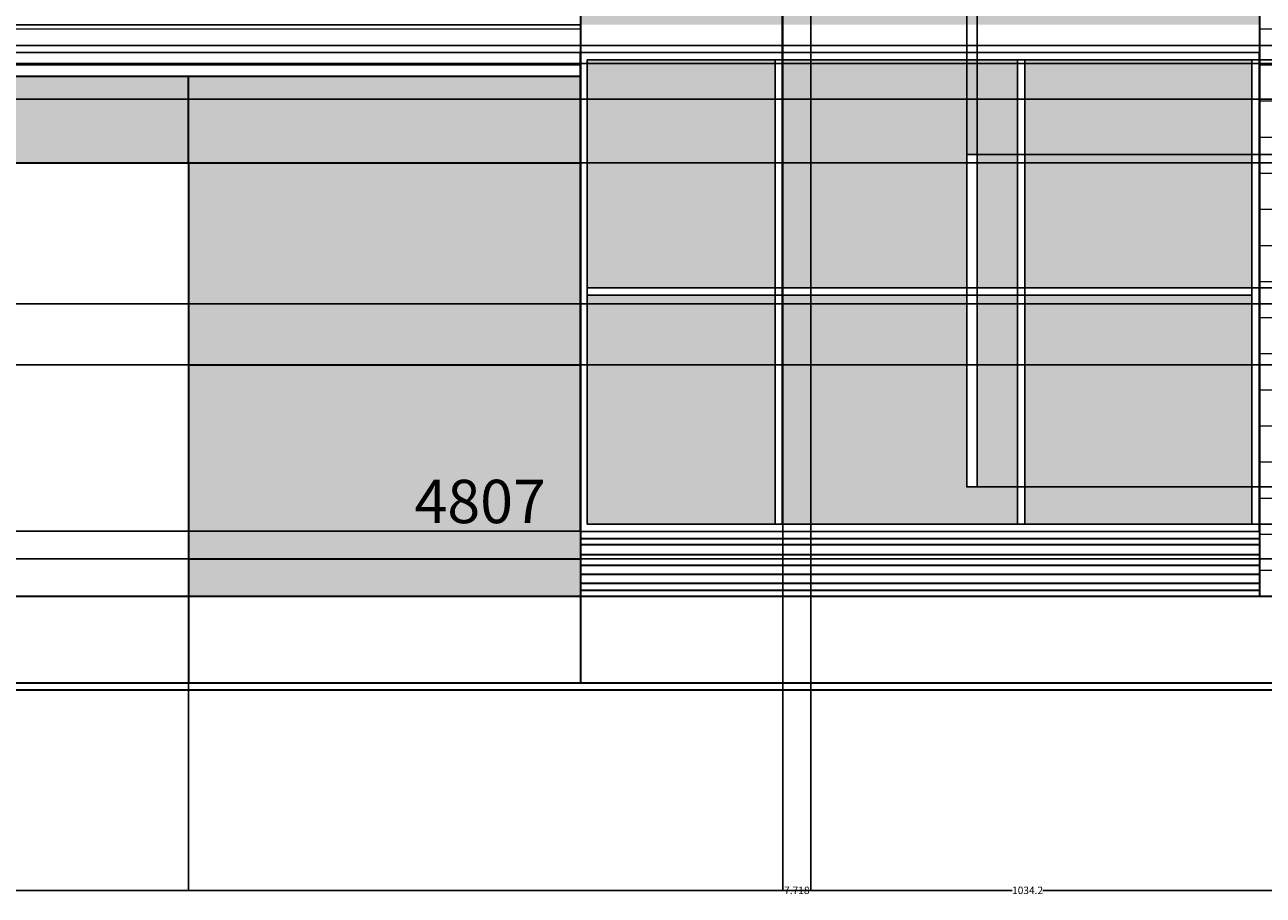
# Model space of a CAD drawing. Units: inches. Extents: x -30 to 1188, y 40 to 520.
# Tile 3 of 7: x 313 to 656, y 40 to 281. Entities that reach past the tile are written whole.
import ezdxf

# ---------------------------------------------------------------- set-up
doc = ezdxf.new("R2010")
doc.units = ezdxf.units.IN
doc.header["$MEASUREMENT"] = 0
for name, color, linetype, lineweight in [('A-ANNO-DIMS', 2, 'Continuous', 18), ('A-ANNO-TEXT', 7, 'Continuous', 25), ('A-DOOR', 3, 'Continuous', 25), ('A-ELEV', 7, 'Continuous', 35), ('A-ELEV-PATT', 8, 'Continuous', 13)]:
    doc.layers.add(name, color=color, linetype=linetype, lineweight=lineweight)
doc.styles.get("Standard").update_dxf_attribs({"font": 'arial.ttf'})
doc.dimstyles.get("Standard").update_dxf_attribs({"dimtxt": 2.0625, "dimasz": 0.18, "dimexe": 0.18, "dimexo": 0.0625, "dimgap": 0.09, "dimtad": 0, "dimtih": 1, "dimtoh": 1, "dimdec": 4, "dimzin": 0, "dimdsep": 46, "dimlunit": 4, "dimtxsty": 'Standard', "dimcen": 0.09, "dimadec": 0, "dimazin": 0, "dimtfac": 1, "dimtdec": 4, "dimtofl": 0, "dimtmove": 0, "dimatfit": 3, "dimfxl": 1, "dimtolj": 1, "dimtzin": 0, "dimarcsym": 0})

# ---------------------------------------------------------------- blocks, each defined once
blk = doc.blocks.new('*D4')
at = {"layer": 'A-ANNO-DIMS', "color": 0, "lineweight": -2, "transparency": 16777216}
for p, q in [((73.66, 122.81), (73.66, 41.19)), ((1107.88, 118.31), (1107.88, 41.19)), ((73.84, 41.37), (586.5, 41.37)), ((1107.7, 41.37), (595.03, 41.37))]:
    blk.add_line(p, q, dxfattribs=at)
at = {"layer": 'A-ANNO-DIMS', "color": 0, "transparency": 16777216}
for points in [[(73.84, 41.4), (73.84, 41.34), (73.66, 41.37)], [(1107.7, 41.4), (1107.7, 41.34), (1107.88, 41.37)]]:
    blk.add_solid(points, dxfattribs=at)
at = {"layer": 'Defpoints', "color": 0, "transparency": 16777216}
for p in [(73.66, 122.87), (1107.88, 118.38), (1107.88, 41.37)]:
    blk.add_point(p, dxfattribs=at)
at = {"layer": 'A-ANNO-DIMS', "color": 0, "transparency": 16777216, "insert": (590.77, 41.37), "char_height": 2.062, "attachment_point": 5}
blk.add_mtext('\\A1;1034.2', dxfattribs=at)
blk = doc.blocks.new('*D9')
at = {"layer": 'A-ANNO-DIMS', "color": 0, "lineweight": -2, "transparency": 16777216}
for p, q in [((99.43, 98.81), (99.43, 41.19)), ((358.42, 98.81), (358.42, 41.19)), ((99.61, 41.37), (226.54, 41.37)), ((358.24, 41.37), (231.32, 41.37))]:
    blk.add_line(p, q, dxfattribs=at)
at = {"layer": 'A-ANNO-DIMS', "color": 0, "transparency": 16777216}
for points in [[(99.61, 41.4), (99.61, 41.34), (99.43, 41.37)], [(358.24, 41.4), (358.24, 41.34), (358.42, 41.37)]]:
    blk.add_solid(points, dxfattribs=at)
at = {"layer": 'Defpoints', "color": 0, "transparency": 16777216}
for p in [(99.43, 98.87), (358.42, 98.87), (358.42, 41.37)]:
    blk.add_point(p, dxfattribs=at)
at = {"layer": 'A-ANNO-DIMS', "color": 0, "transparency": 16777216, "insert": (228.93, 41.37), "char_height": 2.062, "attachment_point": 5}
blk.add_mtext('\\A1;259', dxfattribs=at)
blk = doc.blocks.new('*D20')
at = {"layer": 'A-ANNO-DIMS', "color": 0, "lineweight": -2, "transparency": 16777216}
for p, q in [((358.36, 242.87), (-25.83, 242.87)), ((-25.65, 242.69), (-25.65, 172)), ((-25.65, 99.05), (-25.65, 169.75)), ((358.36, 98.87), (-25.83, 98.87))]:
    blk.add_line(p, q, dxfattribs=at)
at = {"layer": 'A-ANNO-DIMS', "color": 0, "transparency": 16777216}
for points in [[(-25.68, 242.69), (-25.62, 242.69), (-25.65, 242.87)], [(-25.68, 99.05), (-25.62, 99.05), (-25.65, 98.87)]]:
    blk.add_solid(points, dxfattribs=at)
at = {"layer": 'Defpoints', "color": 0, "transparency": 16777216}
for p in [(-25.65, 242.87), (358.42, 242.87), (358.42, 98.87)]:
    blk.add_point(p, dxfattribs=at)
at = {"layer": 'A-ANNO-DIMS', "color": 0, "transparency": 16777216, "insert": (-25.65, 170.87), "char_height": 2.062, "attachment_point": 5}
blk.add_mtext('\\A1;144', dxfattribs=at)
blk = doc.blocks.new('*D29')
at = {"layer": 'A-ANNO-DIMS', "color": 0, "lineweight": -2, "transparency": 16777216}
for p, q in [((792.57, 270.37), (-25.83, 270.37)), ((-25.65, 270.19), (-25.65, 238.25)), ((-25.65, 204.02), (-25.65, 235.96)), ((792.57, 203.84), (-25.83, 203.84))]:
    blk.add_line(p, q, dxfattribs=at)
at = {"layer": 'A-ANNO-DIMS', "color": 0, "transparency": 16777216}
for points in [[(-25.68, 270.19), (-25.62, 270.19), (-25.65, 270.37)], [(-25.68, 204.02), (-25.62, 204.02), (-25.65, 203.84)]]:
    blk.add_solid(points, dxfattribs=at)
at = {"layer": 'Defpoints', "color": 0, "transparency": 16777216}
for p in [(-25.65, 270.37), (792.63, 270.37), (792.63, 203.84)]:
    blk.add_point(p, dxfattribs=at)
at = {"layer": 'A-ANNO-DIMS', "color": 0, "transparency": 16777216, "insert": (-25.65, 237.11), "char_height": 2.062, "attachment_point": 5}
blk.add_mtext('\\A1;66.53', dxfattribs=at)
blk = doc.blocks.new('*D31')
at = {"layer": 'A-ANNO-DIMS', "color": 0, "lineweight": -2, "transparency": 16777216}
for p, q in [((792.57, 203.84), (-25.83, 203.84)), ((-25.65, 203.66), (-25.65, 164.5)), ((-25.65, 123.05), (-25.65, 162.21)), ((935.84, 122.87), (-25.83, 122.87))]:
    blk.add_line(p, q, dxfattribs=at)
at = {"layer": 'A-ANNO-DIMS', "color": 0, "transparency": 16777216}
for points in [[(-25.68, 203.66), (-25.62, 203.66), (-25.65, 203.84)], [(-25.68, 123.05), (-25.62, 123.05), (-25.65, 122.87)]]:
    blk.add_solid(points, dxfattribs=at)
at = {"layer": 'Defpoints', "color": 0, "transparency": 16777216}
for p in [(792.63, 203.84), (-25.65, 122.87), (935.9, 122.87)]:
    blk.add_point(p, dxfattribs=at)
at = {"layer": 'A-ANNO-DIMS', "color": 0, "transparency": 16777216, "insert": (-25.65, 163.36), "char_height": 2.062, "attachment_point": 5}
blk.add_mtext('\\A1;80.97', dxfattribs=at)
blk = doc.blocks.new('*D35')
at = {"layer": 'A-ANNO-DIMS', "color": 0, "lineweight": -2, "transparency": 16777216}
for p, q in [((99.49, 122.87), (1183.93, 122.87)), ((1183.75, 122.69), (1183.75, 112)), ((1183.75, 99.05), (1183.75, 109.75)), ((99.49, 98.87), (1183.93, 98.87))]:
    blk.add_line(p, q, dxfattribs=at)
at = {"layer": 'A-ANNO-DIMS', "color": 0, "transparency": 16777216}
for points in [[(1183.72, 122.69), (1183.78, 122.69), (1183.75, 122.87)], [(1183.72, 99.05), (1183.78, 99.05), (1183.75, 98.87)]]:
    blk.add_solid(points, dxfattribs=at)
at = {"layer": 'Defpoints', "color": 0, "transparency": 16777216}
for p in [(99.43, 122.87), (1183.75, 122.87), (99.43, 98.87)]:
    blk.add_point(p, dxfattribs=at)
at = {"layer": 'A-ANNO-DIMS', "color": 0, "transparency": 16777216, "insert": (1183.75, 110.87), "char_height": 2.062, "attachment_point": 5}
blk.add_mtext('\\A1;24', dxfattribs=at)
blk = doc.blocks.new('*D36')
at = {"layer": 'A-ANNO-DIMS', "color": 0, "lineweight": -2, "transparency": 16777216}
for p, q in [((99.49, 133.14), (1183.93, 133.14)), ((1183.75, 132.96), (1183.75, 129.15)), ((1183.75, 123.05), (1183.75, 126.86)), ((99.49, 122.87), (1183.93, 122.87))]:
    blk.add_line(p, q, dxfattribs=at)
at = {"layer": 'A-ANNO-DIMS', "color": 0, "transparency": 16777216}
for points in [[(1183.72, 132.96), (1183.78, 132.96), (1183.75, 133.14)], [(1183.72, 123.05), (1183.78, 123.05), (1183.75, 122.87)]]:
    blk.add_solid(points, dxfattribs=at)
at = {"layer": 'Defpoints', "color": 0, "transparency": 16777216}
for p in [(99.43, 133.14), (1183.75, 133.14), (99.43, 122.87)]:
    blk.add_point(p, dxfattribs=at)
at = {"layer": 'A-ANNO-DIMS', "color": 0, "transparency": 16777216, "insert": (1183.75, 128.01), "char_height": 2.062, "attachment_point": 5}
blk.add_mtext('\\A1;10.268', dxfattribs=at)
blk = doc.blocks.new('*D37')
at = {"layer": 'A-ANNO-DIMS', "color": 0, "lineweight": -2, "transparency": 16777216}
for p, q in [((99.49, 186.93), (1183.93, 186.93)), ((1183.75, 186.75), (1183.75, 161.18)), ((1183.75, 133.32), (1183.75, 158.89)), ((99.49, 133.14), (1183.93, 133.14))]:
    blk.add_line(p, q, dxfattribs=at)
at = {"layer": 'A-ANNO-DIMS', "color": 0, "transparency": 16777216}
for points in [[(1183.72, 186.75), (1183.78, 186.75), (1183.75, 186.93)], [(1183.72, 133.32), (1183.78, 133.32), (1183.75, 133.14)]]:
    blk.add_solid(points, dxfattribs=at)
at = {"layer": 'Defpoints', "color": 0, "transparency": 16777216}
for p in [(99.43, 186.93), (1183.75, 186.93), (99.43, 133.14)]:
    blk.add_point(p, dxfattribs=at)
at = {"layer": 'A-ANNO-DIMS', "color": 0, "transparency": 16777216, "insert": (1183.75, 160.03), "char_height": 2.062, "attachment_point": 5}
blk.add_mtext('\\A1;53.79', dxfattribs=at)
blk = doc.blocks.new('*D38')
at = {"layer": 'A-ANNO-DIMS', "color": 0, "lineweight": -2, "transparency": 16777216}
for p, q in [((99.49, 242.87), (1183.93, 242.87)), ((1183.75, 242.69), (1183.75, 216.04)), ((1183.75, 187.11), (1183.75, 213.76)), ((99.49, 186.93), (1183.93, 186.93))]:
    blk.add_line(p, q, dxfattribs=at)
at = {"layer": 'A-ANNO-DIMS', "color": 0, "transparency": 16777216}
for points in [[(1183.72, 242.69), (1183.78, 242.69), (1183.75, 242.87)], [(1183.72, 187.11), (1183.78, 187.11), (1183.75, 186.93)]]:
    blk.add_solid(points, dxfattribs=at)
at = {"layer": 'Defpoints', "color": 0, "transparency": 16777216}
for p in [(99.43, 242.87), (1183.75, 242.87), (99.43, 186.93)]:
    blk.add_point(p, dxfattribs=at)
at = {"layer": 'A-ANNO-DIMS', "color": 0, "transparency": 16777216, "insert": (1183.75, 214.9), "char_height": 2.062, "attachment_point": 5}
blk.add_mtext('\\A1;55.94', dxfattribs=at)
blk = doc.blocks.new('*D39')
at = {"layer": 'A-ANNO-DIMS', "color": 0, "lineweight": -2, "transparency": 16777216}
for p, q in [((358.49, 186.93), (1183.93, 186.93)), ((1183.75, 186.75), (1183.75, 161.18)), ((1183.75, 133.32), (1183.75, 158.89)), ((358.49, 133.14), (1183.93, 133.14))]:
    blk.add_line(p, q, dxfattribs=at)
at = {"layer": 'A-ANNO-DIMS', "color": 0, "transparency": 16777216}
for points in [[(1183.72, 186.75), (1183.78, 186.75), (1183.75, 186.93)], [(1183.72, 133.32), (1183.78, 133.32), (1183.75, 133.14)]]:
    blk.add_solid(points, dxfattribs=at)
at = {"layer": 'Defpoints', "color": 0, "transparency": 16777216}
for p in [(358.42, 186.93), (1183.75, 186.93), (358.42, 133.14)]:
    blk.add_point(p, dxfattribs=at)
at = {"layer": 'A-ANNO-DIMS', "color": 0, "transparency": 16777216, "insert": (1183.75, 160.03), "char_height": 2.062, "attachment_point": 5}
blk.add_mtext('\\A1;53.79', dxfattribs=at)
blk = doc.blocks.new('*D40')
at = {"layer": 'A-ANNO-DIMS', "color": 0, "lineweight": -2, "transparency": 16777216}
for p, q in [((358.49, 242.87), (1183.93, 242.87)), ((1183.75, 242.69), (1183.75, 216.04)), ((1183.75, 187.11), (1183.75, 213.76)), ((358.49, 186.93), (1183.93, 186.93))]:
    blk.add_line(p, q, dxfattribs=at)
at = {"layer": 'A-ANNO-DIMS', "color": 0, "transparency": 16777216}
for points in [[(1183.72, 242.69), (1183.78, 242.69), (1183.75, 242.87)], [(1183.72, 187.11), (1183.78, 187.11), (1183.75, 186.93)]]:
    blk.add_solid(points, dxfattribs=at)
at = {"layer": 'Defpoints', "color": 0, "transparency": 16777216}
for p in [(358.42, 242.87), (1183.75, 242.87), (358.42, 186.93)]:
    blk.add_point(p, dxfattribs=at)
at = {"layer": 'A-ANNO-DIMS', "color": 0, "transparency": 16777216, "insert": (1183.75, 214.9), "char_height": 2.062, "attachment_point": 5}
blk.add_mtext('\\A1;55.94', dxfattribs=at)
blk = doc.blocks.new('*D44')
at = {"layer": 'A-ANNO-DIMS', "color": 0, "lineweight": -2, "transparency": 16777216}
for p, q in [((980.66, 275.34), (-25.83, 275.34)), ((-25.65, 275.16), (-25.65, 269.06)), ((-25.65, 260.67), (-25.65, 266.77)), ((980.66, 260.49), (-25.83, 260.49))]:
    blk.add_line(p, q, dxfattribs=at)
at = {"layer": 'A-ANNO-DIMS', "color": 0, "transparency": 16777216}
for points in [[(-25.68, 275.16), (-25.62, 275.16), (-25.65, 275.34)], [(-25.68, 260.67), (-25.62, 260.67), (-25.65, 260.49)]]:
    blk.add_solid(points, dxfattribs=at)
at = {"layer": 'Defpoints', "color": 0, "transparency": 16777216}
for p in [(-25.65, 275.34), (980.73, 275.34), (980.73, 260.49)]:
    blk.add_point(p, dxfattribs=at)
at = {"layer": 'A-ANNO-DIMS', "color": 0, "transparency": 16777216, "insert": (-25.65, 267.92), "char_height": 2.062, "attachment_point": 5}
blk.add_mtext('\\A1;14.85', dxfattribs=at)
blk = doc.blocks.new('*D45')
at = {"layer": 'A-ANNO-DIMS', "color": 0, "lineweight": -2, "transparency": 16777216}
for p, q in [((945.03, 284.84), (-25.83, 284.84)), ((-25.65, 284.66), (-25.65, 273.81)), ((-25.65, 260.67), (-25.65, 271.52)), ((935.84, 260.49), (-25.83, 260.49))]:
    blk.add_line(p, q, dxfattribs=at)
at = {"layer": 'A-ANNO-DIMS', "color": 0, "transparency": 16777216}
for points in [[(-25.68, 284.66), (-25.62, 284.66), (-25.65, 284.84)], [(-25.68, 260.67), (-25.62, 260.67), (-25.65, 260.49)]]:
    blk.add_solid(points, dxfattribs=at)
at = {"layer": 'Defpoints', "color": 0, "transparency": 16777216}
for p in [(945.1, 284.84), (-25.65, 260.49), (935.9, 260.49)]:
    blk.add_point(p, dxfattribs=at)
at = {"layer": 'A-ANNO-DIMS', "color": 0, "transparency": 16777216, "insert": (-25.65, 272.67), "char_height": 2.062, "attachment_point": 5}
blk.add_mtext('\\A1;24.35', dxfattribs=at)
blk = doc.blocks.new('*D55')
at = {"layer": 'A-ANNO-DIMS', "color": 0, "lineweight": -2, "transparency": 16777216}
for p, q in [((466.76, 140.8), (-25.83, 140.8)), ((-25.65, 140.62), (-25.65, 132.98)), ((-25.65, 123.05), (-25.65, 130.69)), ((466.93, 122.87), (-25.83, 122.87))]:
    blk.add_line(p, q, dxfattribs=at)
at = {"layer": 'A-ANNO-DIMS', "color": 0, "transparency": 16777216}
for points in [[(-25.68, 140.62), (-25.62, 140.62), (-25.65, 140.8)], [(-25.68, 123.05), (-25.62, 123.05), (-25.65, 122.87)]]:
    blk.add_solid(points, dxfattribs=at)
at = {"layer": 'Defpoints', "color": 0, "transparency": 16777216}
for p in [(-25.65, 140.8), (466.83, 140.8), (467, 122.87)]:
    blk.add_point(p, dxfattribs=at)
at = {"layer": 'A-ANNO-DIMS', "color": 0, "transparency": 16777216, "insert": (-25.65, 131.83), "char_height": 2.062, "attachment_point": 5}
blk.add_mtext('\\A1;17.927', dxfattribs=at)
blk = doc.blocks.new('*D56')
at = {"layer": 'A-ANNO-DIMS', "color": 0, "lineweight": -2, "transparency": 16777216}
for p, q in [((466.76, 273.38), (-25.83, 273.38)), ((-25.65, 273.2), (-25.65, 208.23)), ((-25.65, 140.98), (-25.65, 205.94)), ((466.76, 140.8), (-25.83, 140.8))]:
    blk.add_line(p, q, dxfattribs=at)
at = {"layer": 'A-ANNO-DIMS', "color": 0, "transparency": 16777216}
for points in [[(-25.68, 273.2), (-25.62, 273.2), (-25.65, 273.38)], [(-25.68, 140.98), (-25.62, 140.98), (-25.65, 140.8)]]:
    blk.add_solid(points, dxfattribs=at)
at = {"layer": 'Defpoints', "color": 0, "transparency": 16777216}
for p in [(-25.65, 273.38), (466.83, 273.38), (466.83, 140.8)]:
    blk.add_point(p, dxfattribs=at)
at = {"layer": 'A-ANNO-DIMS', "color": 0, "transparency": 16777216, "insert": (-25.65, 207.09), "char_height": 2.062, "attachment_point": 5}
blk.add_mtext('\\A1;132.58', dxfattribs=at)
blk = doc.blocks.new('*D57')
at = {"layer": 'A-ANNO-DIMS', "color": 0, "lineweight": -2, "transparency": 16777216}
for p, q in [((466.93, 281.09), (-25.83, 281.09)), ((-25.65, 280.91), (-25.65, 278.38)), ((-25.65, 273.56), (-25.65, 276.09)), ((466.76, 273.38), (-25.83, 273.38))]:
    blk.add_line(p, q, dxfattribs=at)
at = {"layer": 'A-ANNO-DIMS', "color": 0, "transparency": 16777216}
for points in [[(-25.68, 280.91), (-25.62, 280.91), (-25.65, 281.09)], [(-25.68, 273.56), (-25.62, 273.56), (-25.65, 273.38)]]:
    blk.add_solid(points, dxfattribs=at)
at = {"layer": 'Defpoints', "color": 0, "transparency": 16777216}
for p in [(-25.65, 281.09), (467, 281.09), (466.83, 273.38)]:
    blk.add_point(p, dxfattribs=at)
at = {"layer": 'A-ANNO-DIMS', "color": 0, "transparency": 16777216, "insert": (-25.65, 277.23), "char_height": 2.062, "attachment_point": 5}
blk.add_mtext('\\A1;7.718', dxfattribs=at)
blk = doc.blocks.new('*D58')
at = {"layer": 'A-ANNO-DIMS', "color": 0, "lineweight": -2, "transparency": 16777216}
for p, q in [((466.93, 303.05), (-25.83, 303.05)), ((-25.65, 302.87), (-25.65, 293.22)), ((-25.65, 281.27), (-25.65, 290.93)), ((466.93, 281.09), (-25.83, 281.09))]:
    blk.add_line(p, q, dxfattribs=at)
at = {"layer": 'A-ANNO-DIMS', "color": 0, "transparency": 16777216}
for points in [[(-25.68, 302.87), (-25.62, 302.87), (-25.65, 303.05)], [(-25.68, 281.27), (-25.62, 281.27), (-25.65, 281.09)]]:
    blk.add_solid(points, dxfattribs=at)
at = {"layer": 'Defpoints', "color": 0, "transparency": 16777216}
for p in [(-25.65, 303.05), (467, 303.05), (467, 281.09)]:
    blk.add_point(p, dxfattribs=at)
at = {"layer": 'A-ANNO-DIMS', "color": 0, "transparency": 16777216, "insert": (-25.65, 292.07), "char_height": 2.062, "attachment_point": 5}
blk.add_mtext('\\A1;21.96', dxfattribs=at)
blk = doc.blocks.new('*D61')
at = {"layer": 'A-ANNO-DIMS', "color": 0, "lineweight": -2, "transparency": 16777216}
for p, q in [((653.09, 208.22), (1183.93, 208.22)), ((1183.75, 208.04), (1183.75, 176.65)), ((1183.75, 142.98), (1183.75, 174.36)), ((652.92, 142.8), (1183.93, 142.8))]:
    blk.add_line(p, q, dxfattribs=at)
at = {"layer": 'A-ANNO-DIMS', "color": 0, "transparency": 16777216}
for points in [[(1183.72, 208.04), (1183.78, 208.04), (1183.75, 208.22)], [(1183.72, 142.98), (1183.78, 142.98), (1183.75, 142.8)]]:
    blk.add_solid(points, dxfattribs=at)
at = {"layer": 'Defpoints', "color": 0, "transparency": 16777216}
for p in [(653.03, 208.22), (1183.75, 208.22), (652.86, 142.8)]:
    blk.add_point(p, dxfattribs=at)
at = {"layer": 'A-ANNO-DIMS', "color": 0, "transparency": 16777216, "insert": (1183.75, 175.51), "char_height": 2.062, "attachment_point": 5}
blk.add_mtext('\\A1;65.42', dxfattribs=at)
blk = doc.blocks.new('*D62')
at = {"layer": 'A-ANNO-DIMS', "color": 0, "lineweight": -2, "transparency": 16777216}
for p, q in [((652.92, 271.38), (1183.93, 271.38)), ((1183.75, 271.2), (1183.75, 240.94)), ((1183.75, 208.4), (1183.75, 238.65)), ((653.09, 208.22), (1183.93, 208.22))]:
    blk.add_line(p, q, dxfattribs=at)
at = {"layer": 'A-ANNO-DIMS', "color": 0, "transparency": 16777216}
for points in [[(1183.72, 271.2), (1183.78, 271.2), (1183.75, 271.38)], [(1183.72, 208.4), (1183.78, 208.4), (1183.75, 208.22)]]:
    blk.add_solid(points, dxfattribs=at)
at = {"layer": 'Defpoints', "color": 0, "transparency": 16777216}
for p in [(652.86, 271.38), (1183.75, 271.38), (653.03, 208.22)]:
    blk.add_point(p, dxfattribs=at)
at = {"layer": 'A-ANNO-DIMS', "color": 0, "transparency": 16777216, "insert": (1183.75, 239.8), "char_height": 2.062, "attachment_point": 5}
blk.add_mtext('\\A1;63.16', dxfattribs=at)
blk = doc.blocks.new('*D63')
at = {"layer": 'A-ANNO-DIMS', "color": 0, "lineweight": -2, "transparency": 16777216}
for p, q in [((576.85, 153.08), (1183.93, 153.08)), ((1183.75, 152.9), (1183.75, 149.08)), ((1183.75, 142.98), (1183.75, 146.8)), ((588.03, 142.8), (1183.93, 142.8))]:
    blk.add_line(p, q, dxfattribs=at)
at = {"layer": 'A-ANNO-DIMS', "color": 0, "transparency": 16777216}
for points in [[(1183.72, 152.9), (1183.78, 152.9), (1183.75, 153.08)], [(1183.72, 142.98), (1183.78, 142.98), (1183.75, 142.8)]]:
    blk.add_solid(points, dxfattribs=at)
at = {"layer": 'Defpoints', "color": 0, "transparency": 16777216}
for p in [(576.78, 153.08), (587.97, 142.8), (1183.75, 142.8)]:
    blk.add_point(p, dxfattribs=at)
at = {"layer": 'A-ANNO-DIMS', "color": 0, "transparency": 16777216, "insert": (1183.75, 147.94), "char_height": 2.062, "attachment_point": 5}
blk.add_mtext('\\A1;10.286', dxfattribs=at)
blk = doc.blocks.new('*D64')
at = {"layer": 'A-ANNO-DIMS', "color": 0, "lineweight": -2, "transparency": 16777216}
for p, q in [((576.85, 245.17), (1183.93, 245.17)), ((1183.75, 244.99), (1183.75, 200.27)), ((1183.75, 153.26), (1183.75, 197.98)), ((576.85, 153.08), (1183.93, 153.08))]:
    blk.add_line(p, q, dxfattribs=at)
at = {"layer": 'A-ANNO-DIMS', "color": 0, "transparency": 16777216}
for points in [[(1183.72, 244.99), (1183.78, 244.99), (1183.75, 245.17)], [(1183.72, 153.26), (1183.78, 153.26), (1183.75, 153.08)]]:
    blk.add_solid(points, dxfattribs=at)
at = {"layer": 'Defpoints', "color": 0, "transparency": 16777216}
for p in [(576.78, 245.17), (1183.75, 245.17), (576.78, 153.08)]:
    blk.add_point(p, dxfattribs=at)
at = {"layer": 'A-ANNO-DIMS', "color": 0, "transparency": 16777216, "insert": (1183.75, 199.12), "char_height": 2.062, "attachment_point": 5}
blk.add_mtext('\\A1;92.08', dxfattribs=at)
blk = doc.blocks.new('*D65')
at = {"layer": 'A-ANNO-DIMS', "color": 0, "lineweight": -2, "transparency": 16777216}
for p, q in [((522.84, 271.44), (522.84, 518.97)), ((523.02, 518.79), (544.8, 518.79)), ((573.72, 518.79), (551.94, 518.79)), ((573.9, 245.23), (573.9, 518.97))]:
    blk.add_line(p, q, dxfattribs=at)
at = {"layer": 'A-ANNO-DIMS', "color": 0, "transparency": 16777216}
for points in [[(523.02, 518.82), (523.02, 518.76), (522.84, 518.79)], [(573.72, 518.82), (573.72, 518.76), (573.9, 518.79)]]:
    blk.add_solid(points, dxfattribs=at)
at = {"layer": 'Defpoints', "color": 0, "transparency": 16777216}
for p in [(522.84, 518.79), (522.84, 271.38), (573.9, 245.17)]:
    blk.add_point(p, dxfattribs=at)
at = {"layer": 'A-ANNO-DIMS', "color": 0, "transparency": 16777216, "insert": (548.37, 518.79), "char_height": 2.062, "attachment_point": 5}
blk.add_mtext('\\A1;51.07', dxfattribs=at)
blk = doc.blocks.new('*D66')
at = {"layer": 'A-ANNO-DIMS', "color": 0, "lineweight": -2, "transparency": 16777216}
for p, q in [((573.9, 245.23), (573.9, 518.97)), ((574.08, 518.79), (576.6, 518.79)), ((576.78, 245.23), (576.78, 518.97)), ((576.78, 518.79), (576.96, 518.79))]:
    blk.add_line(p, q, dxfattribs=at)
at = {"layer": 'A-ANNO-DIMS', "color": 0, "transparency": 16777216}
for points in [[(574.08, 518.82), (574.08, 518.76), (573.9, 518.79)], [(576.6, 518.82), (576.6, 518.76), (576.78, 518.79)]]:
    blk.add_solid(points, dxfattribs=at)
at = {"layer": 'Defpoints', "color": 0, "transparency": 16777216}
for p in [(576.78, 518.79), (573.9, 245.17), (576.78, 245.17)]:
    blk.add_point(p, dxfattribs=at)
at = {"layer": 'A-ANNO-DIMS', "color": 0, "transparency": 16777216, "insert": (579.75, 518.79), "char_height": 2.062, "attachment_point": 5}
blk.add_mtext('\\A1;2.88', dxfattribs=at)
blk = doc.blocks.new('*D70')
at = {"layer": 'A-ANNO-DIMS', "color": 0, "lineweight": -2, "transparency": 16777216}
for p, q in [((530.73, 332.85), (530.73, 41.19)), ((523.01, 302.99), (523.01, 41.19)), ((523.19, 41.37), (523.3, 41.37)), ((530.55, 41.37), (530.43, 41.37))]:
    blk.add_line(p, q, dxfattribs=at)
at = {"layer": 'A-ANNO-DIMS', "color": 0, "transparency": 16777216}
for points in [[(523.19, 41.4), (523.19, 41.34), (523.01, 41.37)], [(530.55, 41.4), (530.55, 41.34), (530.73, 41.37)]]:
    blk.add_solid(points, dxfattribs=at)
at = {"layer": 'Defpoints', "color": 0, "transparency": 16777216}
for p in [(530.73, 332.91), (523.01, 303.05), (523.01, 41.37)]:
    blk.add_point(p, dxfattribs=at)
at = {"layer": 'A-ANNO-DIMS', "color": 0, "transparency": 16777216, "insert": (526.87, 41.37), "char_height": 2.062, "attachment_point": 5}
blk.add_mtext('\\A1;7.718', dxfattribs=at)
blk = doc.blocks.new('*D74')
at = {"layer": 'A-ANNO-DIMS', "color": 0, "lineweight": -2, "transparency": 16777216}
for p, q in [((30.14, 98.93), (30.14, 518.97)), ((30.32, 518.79), (574.32, 518.79)), ((1128.07, 518.79), (584.07, 518.79)), ((1128.25, 117.62), (1128.25, 518.97))]:
    blk.add_line(p, q, dxfattribs=at)
at = {"layer": 'A-ANNO-DIMS', "color": 0, "transparency": 16777216}
for points in [[(30.32, 518.82), (30.32, 518.76), (30.14, 518.79)], [(1128.07, 518.82), (1128.07, 518.76), (1128.25, 518.79)]]:
    blk.add_solid(points, dxfattribs=at)
at = {"layer": 'Defpoints', "color": 0, "transparency": 16777216}
for p in [(1128.25, 518.79), (1128.25, 117.56), (30.14, 98.87)]:
    blk.add_point(p, dxfattribs=at)
at = {"layer": 'A-ANNO-DIMS', "color": 0, "transparency": 16777216, "insert": (579.19, 518.79), "char_height": 2.0625, "attachment_point": 5}
blk.add_mtext('\\A1;1098.11', dxfattribs=at)

msp = doc.modelspace()

# ---------------------------------------------------------------- hatches: boundary and pattern name
at = {"layer": 'A-ELEV-PATT'}
h = msp.add_hatch(dxfattribs=at)
h.set_pattern_fill('ANSI31', color=256, scale=80, angle=135)
h.paths.add_polyline_path([(935.904, 461.2934), (655.0318, 461.2934), (655.0318, 408.0708), (655.0318, 380.8615), (798.3036, 380.8615), (798.3036, 314.3348), (655.0318, 314.3348), (655.0318, 303.0545), (655.0318, 122.8714), (744.4225, 122.8714), (796.5546, 122.8714), (935.904, 122.8714), (935.904, 203.8438), (792.6322, 203.8438), (792.6322, 270.3705), (935.904, 270.3705), (935.904, 372.8284)])
h.paths.add_polyline_path([(466.9951, 434.8714), (466.9951, 461.2934), (73.6582, 461.2934), (73.6582, 434.8714), (73.6582, 410.8714), (73.6582, 266.8714), (382.4247, 266.8714), (466.9951, 266.8714)])
h.paths.add_polyline_path([(422.6392, 390.3227), (422.6392, 317.8826), (99.4312, 317.8826), (99.4312, 390.3227)], flags=16)
h.paths.add_polyline_path([(416.8376, 385.9009), (416.8376, 322.3026), (332.2885, 322.3026), (332.2885, 385.9009)], flags=0)
h.paths.add_polyline_path([(187.4151, 386.0591), (187.4151, 322.4608), (102.866, 322.4608), (102.866, 386.0591)], flags=0)
h = msp.add_hatch(color=256, dxfattribs=at)
h.dxf.hatch_style = 1
h.paths.add_polyline_path([(99.4312, 186.9265), (73.6582, 186.9265), (73.6582, 133.1393), (99.4312, 133.1393)])
h.paths.add_polyline_path([(99.4312, 242.8714), (73.6582, 242.8714), (73.6582, 186.9265), (99.4312, 186.9265)])
h.paths.add_polyline_path([(99.4312, 266.8714), (73.6582, 266.8714), (73.6582, 242.8714), (99.4312, 242.8714)])
h.paths.add_polyline_path([(244.2768, 266.8714), (99.4312, 266.8714), (99.4312, 242.8714), (130.129, 242.8714), (244.2768, 242.8714)])
h.paths.add_polyline_path([(358.4247, 266.8714), (244.2768, 266.8714), (244.2768, 242.8714), (358.4247, 242.8714)])
h.paths.add_polyline_path([(466.8255, 266.8714), (382.4247, 266.8714), (358.4247, 266.8714), (358.4247, 242.8714), (382.4247, 242.8714), (466.8255, 242.8714)])
h.paths.add_polyline_path([(466.8255, 242.8714), (382.4247, 242.8714), (358.4247, 242.8714), (358.4247, 186.9265), (382.4247, 186.9265), (466.8255, 186.9265)])
h.paths.add_polyline_path([(466.8255, 186.9265), (382.4247, 186.9265), (358.4247, 186.9265), (358.4247, 133.1393), (382.4247, 133.1393), (466.9951, 133.1393), (466.9951, 140.7981), (466.8255, 140.7981)])
h.paths.add_polyline_path([(521.0073, 303.0545), (466.9951, 303.0545), (466.9951, 281.0934), (521.0073, 281.0934)])
h.paths.add_polyline_path([(588.0971, 303.0545), (521.0073, 303.0545), (521.0073, 281.0934), (588.0971, 281.0934)])
h.paths.add_polyline_path([(655.0318, 303.0545), (588.0971, 303.0545), (588.0971, 281.0934), (655.0318, 281.0934)])
h.paths.add_polyline_path([(655.0318, 408.0708), (655.0318, 418.5083), (588.0971, 418.5083), (588.0971, 390.7733), (655.0318, 390.7733)])
h.paths.add_polyline_path([(588.0971, 418.5083), (521.0073, 418.5083), (521.0073, 390.7733), (588.0971, 390.7733)])
h.paths.add_polyline_path([(521.0073, 418.5083), (466.9951, 418.5083), (466.9951, 390.7733), (521.0073, 390.7733)])
h = msp.add_hatch(color=256, dxfattribs=at)
h.dxf.hatch_style = 1
h.paths.add_polyline_path([(237.1312, 390.3227), (187.4151, 390.3227), (187.4151, 386.0591), (187.4151, 322.4608), (187.4151, 317.8826), (237.1312, 317.8826)])
h.paths.add_polyline_path([(289.6973, 390.3227), (237.1312, 390.3227), (237.1312, 317.8826), (289.6973, 317.8826)])
h.paths.add_polyline_path([(422.6392, 390.3227), (289.6973, 390.3227), (289.6973, 317.8826), (422.6392, 317.8826)])
h.paths.add_polyline_path([(332.2885, 385.9009), (416.8376, 385.9009), (416.8376, 322.3026), (332.2885, 322.3026)], flags=16)
h.paths.add_polyline_path([(520.8377, 255.4488), (468.8255, 255.4488), (468.8255, 208.218), (520.8377, 208.218)])
h.paths.add_polyline_path([(573.9028, 245.1654), (576.7826, 245.1654), (576.7826, 208.218), (587.9675, 208.218), (587.9675, 255.4488), (522.8377, 255.4488), (522.8377, 208.218), (573.9028, 208.218)])
h.paths.add_polyline_path([(652.8622, 255.4488), (589.9675, 255.4488), (589.9675, 208.218), (652.8622, 208.218)])
h.paths.add_polyline_path([(652.8622, 206.218), (589.9675, 206.218), (589.9675, 142.7981), (652.8622, 142.7981)])
h.paths.add_polyline_path([(573.9028, 206.218), (522.8377, 206.218), (522.8377, 142.7981), (587.9675, 142.7981), (587.9675, 206.218), (576.7826, 206.218), (576.7826, 153.0843), (573.9028, 153.0843)])
h.paths.add_polyline_path([(520.8377, 206.218), (468.8255, 206.218), (468.8255, 142.7981), (520.8377, 142.7981)])
h.paths.add_polyline_path([(520.8377, 271.3754), (468.8255, 271.3754), (468.8255, 255.4488), (520.8377, 255.4488)])
h.paths.add_polyline_path([(587.9675, 271.3754), (522.8377, 271.3754), (522.8377, 255.4488), (587.9675, 255.4488)])
h.paths.add_polyline_path([(652.8622, 271.3754), (589.9675, 271.3754), (589.9675, 255.4488), (652.8622, 255.4488)])
h.paths.add_polyline_path([(935.904, 270.3705), (886.5164, 270.3705), (886.5164, 268.3705), (886.5164, 205.8438), (886.5164, 203.8438), (935.904, 203.8438)])
h.paths.add_polyline_path([(978.7252, 275.3408), (937.904, 275.3408), (937.904, 262.4906), (978.7252, 262.4906)])
h.paths.add_polyline_path([(978.7252, 370.8284), (937.904, 370.8284), (937.904, 275.3408), (978.7252, 275.3408)])
h.paths.add_polyline_path([(967.928, 284.8425), (945.0964, 284.8425), (945.0964, 357.2748), (967.928, 357.2748)], flags=16)
h = msp.add_hatch(color=256, dxfattribs=at)
h.dxf.hatch_style = 1
h.paths.add_polyline_path([(99.4312, 133.1393), (73.6582, 133.1393), (73.6582, 122.8714), (99.4312, 122.8714)])
h.paths.add_polyline_path([(466.9951, 133.1393), (382.4247, 133.1393), (358.4247, 133.1393), (358.4247, 122.8714), (435.3376, 122.8714), (466.9951, 122.8714)])

# ---------------------------------------------------------------- linework, layer by layer
at = {"layer": 'A-DOOR'}
for p, q in [((520.8377, 271.3754), (520.8377, 142.7981)), ((522.8377, 271.3754), (522.8377, 142.7981)), ((587.9675, 271.3754), (587.9675, 142.7981)), ((589.9675, 271.3754), (589.9675, 142.7981)), ((468.9951, 208.218), (653.0318, 208.218)), ((468.9951, 206.218), (653.0318, 206.218))]:
    msp.add_line(p, q, dxfattribs=at)
for points in [[(466.8255, 273.3754), (654.8622, 273.3754), (654.8622, 140.7981), (466.8255, 140.7981)], [(468.8255, 271.3754), (652.8622, 271.3754), (652.8622, 142.7981), (468.8255, 142.7981)], [(573.9028, 245.1654), (576.7826, 245.1654), (576.7826, 153.0843), (573.9028, 153.0843)]]:
    msp.add_lwpolyline(points, close=True, dxfattribs=at)
at = {"layer": 'A-ELEV'}
for p, q in [((466.9951, 434.8714), (466.9951, 266.8714)), ((655.0318, 408.0708), (655.0318, 122.8714)), ((73.6582, 266.8714), (382.4247, 266.8714)), ((358.4247, 242.8714), (358.4247, 266.8714)), ((382.4247, 266.8714), (466.9951, 266.8714)), ((466.9951, 266.8714), (466.9951, 98.8714)), ((130.129, 242.8714), (358.4247, 242.8714)), ((358.4247, 242.8714), (358.4247, 98.8714)), ((358.4247, 242.8714), (382.4247, 242.8714)), ((382.4247, 242.8714), (466.9951, 242.8714)), ((358.4247, 186.9265), (382.4247, 186.9265)), ((382.4247, 186.9265), (466.9951, 186.9265)), ((466.9951, 138.83), (655.0318, 138.83)), ((466.9951, 137.1922), (655.0318, 137.1922)), ((466.9951, 134.3818), (655.0318, 134.3818)), ((358.4247, 133.1393), (382.4247, 133.1393)), ((382.4247, 133.1393), (466.9951, 133.1393)), ((466.9951, 131.4525), (655.0318, 131.4525)), ((466.9951, 128.9571), (655.0318, 128.9571)), ((466.9951, 126.4618), (655.0318, 126.4618)), ((466.9951, 124.5089), (655.0318, 124.5089)), ((30.1395, 122.8714), (435.3376, 122.8714)), ((435.3376, 122.8714), (466.9951, 122.8714)), ((466.9951, 122.8714), (744.4225, 122.8714)), ((30.1395, 98.8714), (435.3376, 98.8714)), ((30.1395, 96.8714), (435.3376, 96.8714)), ((435.3376, 98.8714), (466.9951, 98.8714)), ((435.3376, 96.8714), (799.1412, 96.8714)), ((466.9951, 98.8714), (799.4646, 98.8714))]:
    msp.add_line(p, q, dxfattribs=at)

# ---------------------------------------------------------------- texts
at = {"layer": 'A-ANNO-TEXT', "insert": (420.9888, 155.0716), "char_height": 12, "attachment_point": 1}
msp.add_mtext_dynamic_manual_height_columns('4807', width=24.276012, gutter_width=1, heights=[0], dxfattribs=at)

# ---------------------------------------------------------------- dimensions: what is measured, and where the dimension line sits
at = {"layer": 'A-ANNO-DIMS'}
for base, p1, p2, override, picture, middle in [((1128.2474, 518.7934), (30.1395, 98.8714), (1128.2474, 117.5588), {"dimdec": 2, "dimlfac": 1, "dimrnd": 0, "dimzin": 0, "dimdsep": 46, "dimlunit": 2}, '*D74', (579.1935, 518.7934)), ((522.8377, 518.7934), (573.9028, 245.1654), (522.8377, 271.3754), {"dimdec": 2, "dimlfac": 1, "dimrnd": 0, "dimzin": 0, "dimdsep": 46, "dimlunit": 2}, '*D65', (548.3702, 518.7934)), ((576.7826, 518.7934), (573.9028, 245.1654), (576.7826, 245.1654), {"dimdec": 2, "dimlfac": 1, "dimrnd": 0, "dimzin": 0, "dimdsep": 46, "dimlunit": 2}, '*D66', (579.751, 518.7934)), ((523.0073, 41.3714), (530.7254, 332.9128), (523.0073, 303.0545), {"dimdec": 3, "dimlfac": 1, "dimrnd": 0, "dimzin": 0, "dimdsep": 46, "dimlunit": 2}, '*D70', (526.8664, 41.3714)), ((1107.8751, 41.3714), (73.6582, 122.8714), (1107.8751, 118.3767), {"dimdec": 1, "dimlfac": 1, "dimrnd": 0, "dimzin": 0, "dimdsep": 46, "dimlunit": 2}, '*D4', (590.7666, 41.3714)), ((358.4247, 41.3714), (99.4312, 98.8714), (358.4247, 98.8714), {"dimdec": 0, "dimlfac": 1, "dimrnd": 0, "dimzin": 0, "dimdsep": 46, "dimlunit": 2}, '*D9', (228.9279, 41.3714))]:
    dim = msp.add_linear_dim(base=base, p1=p1, p2=p2, dimstyle='Standard', override=override, dxfattribs=at)
    dim.commit()
    dim.dimension.update_dxf_attribs({"geometry": picture, "text_midpoint": middle})
for base, p1, p2, override, picture, middle in [((-25.6484, 303.0545), (466.9951, 281.0934), (466.9951, 303.0545), {"dimdec": 2, "dimlfac": 1, "dimrnd": 0, "dimzin": 0, "dimdsep": 46, "dimlunit": 2}, '*D58', (-25.6484, 292.074)), ((-25.6484, 260.4906), (945.0964, 284.8425), (935.904, 260.4906), {"dimdec": 2, "dimlfac": 1, "dimrnd": 0, "dimzin": 0, "dimdsep": 46, "dimlunit": 2}, '*D45', (-25.6484, 272.6666)), ((-25.6484, 281.0934), (466.8255, 273.3754), (466.9951, 281.0934), {"dimdec": 3, "dimlfac": 1, "dimrnd": 0, "dimzin": 0, "dimdsep": 46, "dimlunit": 2}, '*D57', (-25.6484, 277.2344)), ((-25.6484, 275.3408), (980.7252, 260.4906), (980.7252, 275.3408), {"dimdec": 2, "dimlfac": 1, "dimrnd": 0, "dimzin": 0, "dimdsep": 46, "dimlunit": 2}, '*D44', (-25.6484, 267.9157)), ((-25.6484, 273.3754), (466.8255, 140.7981), (466.8255, 273.3754), {"dimdec": 2, "dimlfac": 1, "dimrnd": 0, "dimzin": 0, "dimdsep": 46, "dimlunit": 2}, '*D56', (-25.6484, 207.0867)), ((1183.7474, 271.3754), (653.0318, 208.218), (652.8622, 271.3754), {"dimdec": 2, "dimlfac": 1, "dimrnd": 0, "dimzin": 0, "dimdsep": 46, "dimlunit": 2}, '*D62', (1183.7474, 239.7967)), ((-25.6484, 270.3705), (792.6322, 203.8438), (792.6322, 270.3705), {"dimdec": 2, "dimlfac": 1, "dimrnd": 0, "dimzin": 0, "dimdsep": 46, "dimlunit": 2}, '*D29', (-25.6484, 237.1071)), ((1183.7474, 245.1654), (576.7826, 153.0843), (576.7826, 245.1654), {"dimdec": 2, "dimlfac": 1, "dimrnd": 0, "dimzin": 0, "dimdsep": 46, "dimlunit": 2}, '*D64', (1183.7474, 199.1248)), ((-25.6484, 242.8714), (358.4247, 98.8714), (358.4247, 242.8714), {"dimdec": 0, "dimlfac": 1, "dimrnd": 0, "dimzin": 0, "dimdsep": 46, "dimlunit": 2}, '*D20', (-25.6484, 170.8714)), ((1183.7474, 242.8714), (99.4312, 186.9265), (99.4312, 242.8714), {"dimdec": 2, "dimlfac": 1, "dimrnd": 0, "dimzin": 0, "dimdsep": 46, "dimlunit": 2}, '*D38', (1183.7474, 214.899)), ((1183.7474, 242.8714), (358.4247, 186.9265), (358.4247, 242.8714), {"dimdec": 2, "dimlfac": 1, "dimrnd": 0, "dimzin": 0, "dimdsep": 46, "dimlunit": 2}, '*D40', (1183.7474, 214.899)), ((1183.7474, 208.218), (652.8622, 142.7981), (653.0318, 208.218), {"dimdec": 2, "dimlfac": 1, "dimrnd": 0, "dimzin": 0, "dimdsep": 46, "dimlunit": 2}, '*D61', (1183.7474, 175.508)), ((-25.6484, 122.8714), (792.6322, 203.8438), (935.904, 122.8714), {"dimdec": 2, "dimlfac": 1, "dimrnd": 0, "dimzin": 0, "dimdsep": 46, "dimlunit": 2}, '*D31', (-25.6484, 163.3576)), ((1183.7474, 186.9265), (99.4312, 133.1393), (99.4312, 186.9265), {"dimdec": 2, "dimlfac": 1, "dimrnd": 0, "dimzin": 0, "dimdsep": 46, "dimlunit": 2}, '*D37', (1183.7474, 160.0329)), ((1183.7474, 186.9265), (358.4247, 133.1393), (358.4247, 186.9265), {"dimdec": 2, "dimlfac": 1, "dimrnd": 0, "dimzin": 0, "dimdsep": 46, "dimlunit": 2}, '*D39', (1183.7474, 160.0329)), ((1183.7474, 142.7981), (576.7826, 153.0843), (587.9675, 142.7981), {"dimdec": 3, "dimlfac": 1, "dimrnd": 0, "dimzin": 0, "dimdsep": 46, "dimlunit": 2}, '*D63', (1183.7474, 147.9412)), ((-25.6484, 140.7981), (466.9951, 122.8714), (466.8255, 140.7981), {"dimdec": 3, "dimlfac": 1, "dimrnd": 0, "dimzin": 0, "dimdsep": 46, "dimlunit": 2}, '*D55', (-25.6484, 131.8348)), ((1183.7474, 133.1393), (99.4312, 122.8714), (99.4312, 133.1393), {"dimdec": 3, "dimlfac": 1, "dimrnd": 0, "dimzin": 0, "dimdsep": 46, "dimlunit": 2}, '*D36', (1183.7474, 128.0054)), ((1183.7474, 122.8714), (99.4312, 98.8714), (99.4312, 122.8714), {"dimdec": 0, "dimlfac": 1, "dimrnd": 0, "dimzin": 0, "dimdsep": 46, "dimlunit": 2}, '*D35', (1183.7474, 110.8714))]:
    dim = msp.add_linear_dim(base=base, p1=p1, p2=p2, angle=90, dimstyle='Standard', override=override, dxfattribs=at)
    dim.commit()
    dim.dimension.update_dxf_attribs({"geometry": picture, "text_midpoint": middle})

doc.saveas('drawing.dxf')
